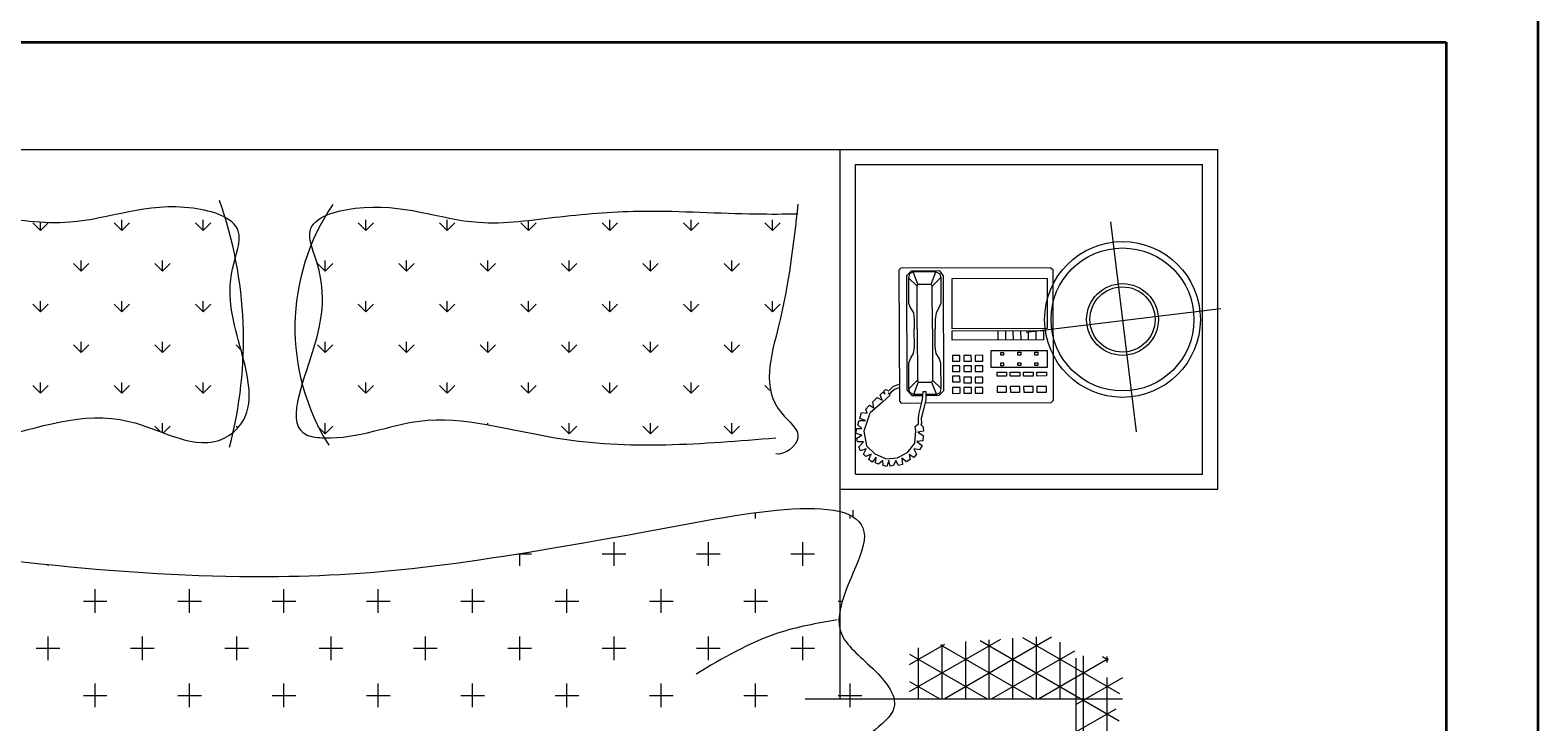
# Model space of a CAD drawing. Units: inches. Extents: x 3731 to 4318, y 1310 to 2388.
# Tile 55 of 57: x 4157 to 4239, y 2296 to 2334. Entities that reach past the tile are written whole.
import ezdxf

# ---------------------------------------------------------------- set-up
doc = ezdxf.new("R2010")
doc.units = ezdxf.units.IN
for name, color, linetype, lineweight in [('A-ANNO-DIMS', 2, 'Continuous', 18), ('A-FURN', 8, 'Continuous', 13), ('A-WALL', 7, 'Continuous', 35)]:
    doc.layers.add(name, color=color, linetype=linetype, lineweight=lineweight)
doc.styles.get("Standard").update_dxf_attribs({"font": 'arial.ttf'})
doc.dimstyles.get("Standard").update_dxf_attribs({"dimtxt": 0.18, "dimasz": 0.18, "dimexe": 0.18, "dimexo": 0.0625, "dimgap": 0.09, "dimtad": 0, "dimtih": 1, "dimtoh": 1, "dimdec": 4, "dimzin": 0, "dimdsep": 46, "dimtxsty": 'Standard', "dimcen": 0.09, "dimadec": 0, "dimazin": 0, "dimtfac": 1, "dimtdec": 4, "dimtofl": 0, "dimtmove": 0, "dimatfit": 3, "dimfxl": 1, "dimtolj": 1, "dimtzin": 0, "dimarcsym": 0})

# ---------------------------------------------------------------- blocks, each defined once
blk = doc.blocks.new('A$C200C7901')
for p, q in [((0.5, 2.3334), (2, 2.3334)), ((2, 2.3334), (2.5, 2.3334)), ((2, 1.6055), (2, 2.3334)), ((2.5, 1.8834), (2.5, 2.3334)), ((0.9943, 2.1721), (0.9842, 2.1822)), ((0.9943, 2.1721), (0.9842, 2.1822)), ((1.3176, 2.1721), (1.3075, 2.1822)), ((1.3176, 2.1721), (1.3075, 2.1822)), ((0.9943, 2.0643), (0.9842, 2.0744)), ((0.9943, 2.0643), (0.9842, 2.0744)), ((1.206, 2.0681), (1.1997, 2.0744)), ((1.206, 2.0681), (1.1997, 2.0744)), ((1.2019, 1.9645), (1.1997, 1.9666)), ((1.2019, 1.9645), (1.1997, 1.9666)), ((2, 1.8834), (2.5, 1.8834)), ((2.0129, 1.8445), (2.0129, 1.849)), ((2.0129, 1.8445), (2.0129, 1.849)), ((2.0171, 1.8467), (2.0171, 1.8556)), ((2.0171, 1.8467), (2.0171, 1.8556)), ((1.1379, 1.7195), (1.1379, 1.7508)), ((1.1222, 1.7352), (1.1535, 1.7352)), ((1.9972, 1.7352), (2.0027, 1.7352)), ((1.9972, 1.7352), (2.0027, 1.7352)), ((2, 1.6963), (2, 1.7248)), ((2, 1.6963), (2, 1.7248)), ((2.3121, 1.6596), (2.3121, 0.0201)), ((1.0129, 1.5945), (1.0129, 1.6258)), ((1.0129, 1.5945), (1.0129, 1.6258)), ((1.9533, 1.6055), (2.3741, 1.6055)), ((1.9533, 1.6055), (2.3741, 1.6055))]:
    blk.add_line(p, q)
at = {"linetype": 'ByBlock'}
for p, q in [((2.02, 2.3134), (2.48, 2.3134)), ((2.02, 1.9034), (2.02, 2.3134)), ((2.48, 1.9034), (2.48, 2.3134)), ((1.0482, 2.2259), (1.0482, 2.2402)), ((1.0482, 2.2259), (1.0482, 2.2402)), ((1.1559, 2.2259), (1.1559, 2.2402)), ((1.1559, 2.2259), (1.1559, 2.2402)), ((1.3714, 2.2259), (1.3714, 2.2402)), ((1.3714, 2.2259), (1.3714, 2.2402)), ((1.4792, 2.2259), (1.4792, 2.2402)), ((1.4792, 2.2259), (1.4792, 2.2402)), ((1.587, 2.2259), (1.587, 2.2393)), ((1.587, 2.2259), (1.587, 2.2393)), ((1.6947, 2.2259), (1.6947, 2.2402)), ((1.6947, 2.2259), (1.6947, 2.2402)), ((1.8025, 2.2259), (1.8025, 2.2402)), ((1.8025, 2.2259), (1.8025, 2.2402)), ((1.9103, 2.2259), (1.9103, 2.2402)), ((1.9103, 2.2259), (1.9103, 2.2402)), ((2.3581, 2.2373), (2.3919, 1.9595)), ((0.9404, 2.2259), (0.9303, 2.236)), ((0.9404, 2.2259), (0.9303, 2.236)), ((0.9404, 2.2259), (0.9404, 2.2369)), ((0.9404, 2.2259), (0.9404, 2.2369)), ((0.9404, 2.2259), (0.9505, 2.236)), ((0.9404, 2.2259), (0.9505, 2.236)), ((1.0482, 2.2259), (1.0381, 2.236)), ((1.0482, 2.2259), (1.0381, 2.236)), ((1.0482, 2.2259), (1.0583, 2.236)), ((1.0482, 2.2259), (1.0583, 2.236)), ((1.1559, 2.2259), (1.1458, 2.236)), ((1.1559, 2.2259), (1.1458, 2.236)), ((1.1559, 2.2259), (1.166, 2.236)), ((1.1559, 2.2259), (1.166, 2.236)), ((1.3714, 2.2259), (1.3613, 2.236)), ((1.3714, 2.2259), (1.3613, 2.236)), ((1.3714, 2.2259), (1.3815, 2.236)), ((1.3714, 2.2259), (1.3815, 2.236)), ((1.4792, 2.2259), (1.4691, 2.236)), ((1.4792, 2.2259), (1.4691, 2.236)), ((1.4792, 2.2259), (1.4893, 2.236)), ((1.4792, 2.2259), (1.4893, 2.236)), ((1.587, 2.2259), (1.5769, 2.236)), ((1.587, 2.2259), (1.5769, 2.236)), ((1.587, 2.2259), (1.5971, 2.236)), ((1.587, 2.2259), (1.5971, 2.236)), ((1.6947, 2.2259), (1.6846, 2.236)), ((1.6947, 2.2259), (1.6846, 2.236)), ((1.6947, 2.2259), (1.7048, 2.236)), ((1.6947, 2.2259), (1.7048, 2.236)), ((1.8025, 2.2259), (1.7924, 2.236)), ((1.8025, 2.2259), (1.7924, 2.236)), ((1.8025, 2.2259), (1.8126, 2.236)), ((1.8025, 2.2259), (1.8126, 2.236)), ((1.9103, 2.2259), (1.9002, 2.236)), ((1.9103, 2.2259), (1.9002, 2.236)), ((1.9103, 2.2259), (1.9204, 2.236)), ((1.9103, 2.2259), (1.9204, 2.236)), ((0.9943, 2.172), (0.9943, 2.1863)), ((0.9943, 2.172), (0.9943, 2.1863)), ((0.9943, 2.1721), (1.0044, 2.1822)), ((0.9943, 2.1721), (1.0044, 2.1822)), ((1.102, 2.1721), (1.0919, 2.1822)), ((1.102, 2.1721), (1.0919, 2.1822)), ((1.102, 2.172), (1.102, 2.1863)), ((1.102, 2.172), (1.102, 2.1863)), ((1.102, 2.1721), (1.1121, 2.1822)), ((1.102, 2.1721), (1.1121, 2.1822)), ((1.3176, 2.172), (1.3176, 2.1863)), ((1.3176, 2.172), (1.3176, 2.1863)), ((1.3176, 2.1721), (1.3277, 2.1822)), ((1.3176, 2.1721), (1.3277, 2.1822)), ((1.4253, 2.1721), (1.4152, 2.1822)), ((1.4253, 2.1721), (1.4152, 2.1822)), ((1.4253, 2.172), (1.4253, 2.1863)), ((1.4253, 2.172), (1.4253, 2.1863)), ((1.4253, 2.1721), (1.4354, 2.1822)), ((1.4253, 2.1721), (1.4354, 2.1822)), ((1.5331, 2.1721), (1.523, 2.1822)), ((1.5331, 2.1721), (1.523, 2.1822)), ((1.5331, 2.172), (1.5331, 2.1863)), ((1.5331, 2.172), (1.5331, 2.1863)), ((1.5331, 2.1721), (1.5432, 2.1822)), ((1.5331, 2.1721), (1.5432, 2.1822)), ((1.6409, 2.1721), (1.6308, 2.1822)), ((1.6409, 2.1721), (1.6308, 2.1822)), ((1.6408, 2.172), (1.6408, 2.1863)), ((1.6408, 2.172), (1.6408, 2.1863)), ((1.6409, 2.1721), (1.651, 2.1822)), ((1.6409, 2.1721), (1.651, 2.1822)), ((1.7486, 2.1721), (1.7385, 2.1822)), ((1.7486, 2.1721), (1.7385, 2.1822)), ((1.7486, 2.172), (1.7486, 2.1863)), ((1.7486, 2.172), (1.7486, 2.1863)), ((1.7486, 2.1721), (1.7587, 2.1822)), ((1.7486, 2.1721), (1.7587, 2.1822)), ((1.8564, 2.1721), (1.8463, 2.1822)), ((1.8564, 2.1721), (1.8463, 2.1822)), ((1.8564, 2.172), (1.8564, 2.1863)), ((1.8564, 2.172), (1.8564, 2.1863)), ((1.8564, 2.1721), (1.8665, 2.1822)), ((1.8564, 2.1721), (1.8665, 2.1822)), ((2.0802, 2.176), (2.0777, 2.1734)), ((2.0777, 2.1734), (2.0783, 1.9999)), ((2.2789, 2.1766), (2.0802, 2.176)), ((2.0941, 2.1722), (2.0878, 2.1659)), ((2.0878, 2.1659), (2.0883, 2.015)), ((2.0915, 2.1685), (2.0903, 2.1634)), ((2.0903, 2.1634), (2.1017, 2.1521)), ((2.0903, 2.1634), (2.0904, 2.1295)), ((2.0966, 2.171), (2.0915, 2.1685)), ((2.1318, 2.1724), (2.0941, 2.1722)), ((2.1267, 2.1711), (2.0966, 2.171)), ((2.1029, 2.1547), (2.0966, 2.171)), ((2.1205, 2.1547), (2.1267, 2.1711)), ((2.1331, 2.1636), (2.1218, 2.1522)), ((2.1267, 2.1711), (2.1318, 2.1686)), ((2.1368, 2.1661), (2.1318, 2.1724)), ((2.1318, 2.1686), (2.1331, 2.1636)), ((2.1331, 2.1636), (2.1332, 2.1296)), ((2.1373, 2.014), (2.1368, 2.1661)), ((2.1481, 2.1624), (2.2739, 2.1628)), ((2.1484, 2.0957), (2.1481, 2.1624)), ((2.2739, 2.1628), (2.2741, 2.0961)), ((2.2789, 2.1766), (2.2814, 2.1741)), ((2.2814, 2.1741), (2.282, 2.0006)), ((2.1017, 2.1521), (2.1029, 2.1547)), ((2.1019, 2.0956), (2.1017, 2.1521)), ((2.1029, 2.1547), (2.1205, 2.1547)), ((2.1218, 2.1522), (2.1205, 2.1547)), ((2.122, 2.0956), (2.1218, 2.1522)), ((0.9404, 2.1182), (0.9303, 2.1283)), ((0.9404, 2.1182), (0.9303, 2.1283)), ((0.9404, 2.1182), (0.9404, 2.1325)), ((0.9404, 2.1182), (0.9404, 2.1325)), ((0.9404, 2.1182), (0.9505, 2.1283)), ((0.9404, 2.1182), (0.9505, 2.1283)), ((1.0482, 2.1182), (1.0381, 2.1283)), ((1.0482, 2.1182), (1.0381, 2.1283)), ((1.0482, 2.1182), (1.0482, 2.1325)), ((1.0482, 2.1182), (1.0482, 2.1325)), ((1.0482, 2.1182), (1.0583, 2.1283)), ((1.0482, 2.1182), (1.0583, 2.1283)), ((1.1559, 2.1182), (1.1458, 2.1283)), ((1.1559, 2.1182), (1.1458, 2.1283)), ((1.1559, 2.1182), (1.1559, 2.1325)), ((1.1559, 2.1182), (1.1559, 2.1325)), ((1.1559, 2.1182), (1.166, 2.1283)), ((1.1559, 2.1182), (1.166, 2.1283)), ((1.3714, 2.1182), (1.3613, 2.1283)), ((1.3714, 2.1182), (1.3613, 2.1283)), ((1.3714, 2.1182), (1.3714, 2.1325)), ((1.3714, 2.1182), (1.3714, 2.1325)), ((1.3714, 2.1182), (1.3815, 2.1283)), ((1.3714, 2.1182), (1.3815, 2.1283)), ((1.4792, 2.1182), (1.4691, 2.1283)), ((1.4792, 2.1182), (1.4691, 2.1283)), ((1.4792, 2.1182), (1.4792, 2.1325)), ((1.4792, 2.1182), (1.4792, 2.1325)), ((1.4792, 2.1182), (1.4893, 2.1283)), ((1.4792, 2.1182), (1.4893, 2.1283)), ((1.587, 2.1182), (1.5769, 2.1283)), ((1.587, 2.1182), (1.5769, 2.1283)), ((1.587, 2.1182), (1.587, 2.1325)), ((1.587, 2.1182), (1.587, 2.1325)), ((1.587, 2.1182), (1.5971, 2.1283)), ((1.587, 2.1182), (1.5971, 2.1283)), ((1.6947, 2.1182), (1.6846, 2.1283)), ((1.6947, 2.1182), (1.6846, 2.1283)), ((1.6947, 2.1182), (1.6947, 2.1325)), ((1.6947, 2.1182), (1.6947, 2.1325)), ((1.6947, 2.1182), (1.7048, 2.1283)), ((1.6947, 2.1182), (1.7048, 2.1283)), ((1.8025, 2.1182), (1.7924, 2.1283)), ((1.8025, 2.1182), (1.7924, 2.1283)), ((1.8025, 2.1182), (1.8025, 2.1325)), ((1.8025, 2.1182), (1.8025, 2.1325)), ((1.8025, 2.1182), (1.8126, 2.1283)), ((1.8025, 2.1182), (1.8126, 2.1283)), ((1.9103, 2.1182), (1.9002, 2.1283)), ((1.9103, 2.1182), (1.9002, 2.1283)), ((1.9103, 2.1182), (1.9103, 2.1325)), ((1.9103, 2.1182), (1.9103, 2.1325)), ((1.9103, 2.1182), (1.9204, 2.1283)), ((1.9103, 2.1182), (1.9204, 2.1283)), ((2.0904, 2.1295), (2.093, 2.1232)), ((2.093, 2.1232), (2.0968, 2.1169)), ((2.1307, 2.1233), (2.1269, 2.117)), ((2.1332, 2.1296), (2.1307, 2.1233)), ((2.2464, 2.0911), (2.5044, 2.1228)), ((2.0968, 2.1169), (2.098, 2.1081)), ((2.098, 2.1081), (2.0981, 2.0956)), ((2.1269, 2.117), (2.1257, 2.1082)), ((2.1257, 2.1082), (2.1257, 2.0956)), ((0.9943, 2.0643), (0.9943, 2.0786)), ((0.9943, 2.0643), (0.9943, 2.0786)), ((1.102, 2.0643), (1.102, 2.0786)), ((1.102, 2.0643), (1.102, 2.0786)), ((1.3176, 2.0643), (1.3176, 2.0786)), ((1.3176, 2.0643), (1.3176, 2.0786)), ((1.4253, 2.0643), (1.4253, 2.0786)), ((1.4253, 2.0643), (1.4253, 2.0786)), ((1.5331, 2.0643), (1.5331, 2.0786)), ((1.5331, 2.0643), (1.5331, 2.0786)), ((1.6408, 2.0643), (1.6408, 2.0786)), ((1.6408, 2.0643), (1.6408, 2.0786)), ((1.7486, 2.0643), (1.7486, 2.0786)), ((1.7486, 2.0643), (1.7486, 2.0786)), ((1.8564, 2.0643), (1.8564, 2.0786)), ((1.8564, 2.0643), (1.8564, 2.0786)), ((2.0982, 2.0717), (2.0981, 2.0956)), ((2.1019, 2.0956), (2.1021, 2.0277)), ((2.122, 2.0956), (2.1222, 2.0277)), ((2.1258, 2.0718), (2.1257, 2.0956)), ((2.2741, 2.0961), (2.1484, 2.0957)), ((2.1484, 2.0932), (2.2691, 2.0936)), ((2.1484, 2.0806), (2.1484, 2.0932)), ((2.2691, 2.081), (2.1484, 2.0806)), ((2.2087, 2.0934), (2.2088, 2.0808)), ((2.2188, 2.0934), (2.2188, 2.0809)), ((2.2288, 2.0935), (2.2289, 2.0809)), ((2.2389, 2.0935), (2.239, 2.0809)), ((2.249, 2.0935), (2.249, 2.081)), ((2.259, 2.0936), (2.2591, 2.081)), ((2.2691, 2.0936), (2.2691, 2.081)), ((0.9943, 2.0643), (1.0044, 2.0744)), ((0.9943, 2.0643), (1.0044, 2.0744)), ((1.102, 2.0643), (1.0919, 2.0744)), ((1.102, 2.0643), (1.0919, 2.0744)), ((1.102, 2.0643), (1.1121, 2.0744)), ((1.102, 2.0643), (1.1121, 2.0744)), ((1.3176, 2.0643), (1.3075, 2.0744)), ((1.3176, 2.0643), (1.3075, 2.0744)), ((1.3176, 2.0643), (1.3277, 2.0744)), ((1.3176, 2.0643), (1.3277, 2.0744)), ((1.4253, 2.0643), (1.4152, 2.0744)), ((1.4253, 2.0643), (1.4152, 2.0744)), ((1.4253, 2.0643), (1.4354, 2.0744)), ((1.4253, 2.0643), (1.4354, 2.0744)), ((1.5331, 2.0643), (1.523, 2.0744)), ((1.5331, 2.0643), (1.523, 2.0744)), ((1.5331, 2.0643), (1.5432, 2.0744)), ((1.5331, 2.0643), (1.5432, 2.0744)), ((1.6409, 2.0643), (1.6308, 2.0744)), ((1.6409, 2.0643), (1.6308, 2.0744)), ((1.6409, 2.0643), (1.651, 2.0744)), ((1.6409, 2.0643), (1.651, 2.0744)), ((1.7486, 2.0643), (1.7385, 2.0744)), ((1.7486, 2.0643), (1.7385, 2.0744)), ((1.7486, 2.0643), (1.7587, 2.0744)), ((1.7486, 2.0643), (1.7587, 2.0744)), ((1.8564, 2.0643), (1.8463, 2.0744)), ((1.8564, 2.0643), (1.8463, 2.0744)), ((1.8564, 2.0643), (1.8665, 2.0744)), ((1.8564, 2.0643), (1.8665, 2.0744)), ((2.0932, 2.0566), (2.0969, 2.0629)), ((2.0969, 2.0629), (2.0982, 2.0717)), ((2.1271, 2.063), (2.1258, 2.0718)), ((2.1309, 2.0567), (2.1271, 2.063)), ((2.1586, 2.0606), (2.1485, 2.0605)), ((2.1485, 2.0605), (2.1485, 2.053)), ((2.1586, 2.053), (2.1586, 2.0606)), ((2.1636, 2.0606), (2.1636, 2.053)), ((2.1736, 2.0606), (2.1636, 2.0606)), ((2.1737, 2.0531), (2.1736, 2.0606)), ((2.1887, 2.0607), (2.1787, 2.0606)), ((2.1787, 2.0606), (2.1787, 2.0531)), ((2.1888, 2.0531), (2.1887, 2.0607)), ((2.2, 2.067), (2.2742, 2.0672)), ((2.2001, 2.0443), (2.2, 2.067)), ((2.2126, 2.0645), (2.2164, 2.0645)), ((2.2126, 2.0607), (2.2126, 2.0645)), ((2.2164, 2.0607), (2.2126, 2.0607)), ((2.2164, 2.0645), (2.2164, 2.0607)), ((2.2352, 2.0646), (2.239, 2.0646)), ((2.2352, 2.0608), (2.2352, 2.0646)), ((2.239, 2.0608), (2.2352, 2.0608)), ((2.239, 2.0646), (2.239, 2.0608)), ((2.2579, 2.0609), (2.2579, 2.0647)), ((2.2579, 2.0647), (2.2616, 2.0647)), ((2.2616, 2.0609), (2.2579, 2.0609)), ((2.2616, 2.0647), (2.2616, 2.0609)), ((2.2742, 2.0672), (2.2743, 2.0446)), ((2.0907, 2.0503), (2.0932, 2.0566)), ((2.0908, 2.0163), (2.0907, 2.0503)), ((2.1334, 2.0504), (2.1309, 2.0567)), ((2.1336, 2.0165), (2.1334, 2.0504)), ((2.1485, 2.053), (2.1586, 2.053)), ((2.1485, 2.0467), (2.1486, 2.0391)), ((2.1586, 2.0467), (2.1485, 2.0467)), ((2.1486, 2.0391), (2.1586, 2.0392)), ((2.1586, 2.0392), (2.1586, 2.0467)), ((2.1636, 2.053), (2.1737, 2.0531)), ((2.1737, 2.0468), (2.1636, 2.0467)), ((2.1636, 2.0467), (2.1637, 2.0392)), ((2.1637, 2.0392), (2.1737, 2.0392)), ((2.1737, 2.0392), (2.1737, 2.0468)), ((2.1787, 2.0531), (2.1888, 2.0531)), ((2.1787, 2.0468), (2.1787, 2.0392)), ((2.1888, 2.0468), (2.1787, 2.0468)), ((2.1787, 2.0392), (2.1888, 2.0393)), ((2.1888, 2.0393), (2.1888, 2.0468)), ((2.2743, 2.0446), (2.2001, 2.0443)), ((2.2077, 2.0331), (2.2077, 2.0381)), ((2.2077, 2.0381), (2.2202, 2.0381)), ((2.2126, 2.0507), (2.2164, 2.0507)), ((2.2127, 2.0469), (2.2126, 2.0507)), ((2.2164, 2.0469), (2.2127, 2.0469)), ((2.2164, 2.0507), (2.2164, 2.0469)), ((2.2202, 2.0381), (2.2203, 2.0331)), ((2.2253, 2.0381), (2.2378, 2.0382)), ((2.2253, 2.0331), (2.2253, 2.0381)), ((2.2353, 2.0508), (2.2391, 2.0508)), ((2.2353, 2.047), (2.2353, 2.0508)), ((2.2391, 2.047), (2.2353, 2.047)), ((2.2378, 2.0382), (2.2379, 2.0332)), ((2.2391, 2.0508), (2.2391, 2.047)), ((2.2429, 2.0332), (2.2429, 2.0382)), ((2.2429, 2.0382), (2.2554, 2.0382)), ((2.2554, 2.0382), (2.2555, 2.0332)), ((2.2579, 2.0508), (2.2617, 2.0508)), ((2.2579, 2.0471), (2.2579, 2.0508)), ((2.2617, 2.0471), (2.2579, 2.0471)), ((2.2605, 2.0332), (2.2605, 2.0383)), ((2.2605, 2.0383), (2.273, 2.0383)), ((2.2617, 2.0508), (2.2617, 2.0471)), ((2.273, 2.0383), (2.2731, 2.0333)), ((0.9404, 2.0104), (0.9303, 2.0205)), ((0.9404, 2.0104), (0.9303, 2.0205)), ((0.9404, 2.0104), (0.9404, 2.0247)), ((0.9404, 2.0104), (0.9404, 2.0247)), ((0.9404, 2.0104), (0.9505, 2.0205)), ((0.9404, 2.0104), (0.9505, 2.0205)), ((1.0482, 2.0104), (1.0381, 2.0205)), ((1.0482, 2.0104), (1.0381, 2.0205)), ((1.0482, 2.0104), (1.0482, 2.0247)), ((1.0482, 2.0104), (1.0482, 2.0247)), ((1.0482, 2.0104), (1.0583, 2.0205)), ((1.0482, 2.0104), (1.0583, 2.0205)), ((1.1559, 2.0104), (1.1458, 2.0205)), ((1.1559, 2.0104), (1.1458, 2.0205)), ((1.1559, 2.0104), (1.1559, 2.0247)), ((1.1559, 2.0104), (1.1559, 2.0247)), ((1.1559, 2.0104), (1.166, 2.0205)), ((1.1559, 2.0104), (1.166, 2.0205)), ((1.3714, 2.0104), (1.3613, 2.0205)), ((1.3714, 2.0104), (1.3613, 2.0205)), ((1.3714, 2.0104), (1.3714, 2.0247)), ((1.3714, 2.0104), (1.3714, 2.0247)), ((1.3714, 2.0104), (1.3815, 2.0205)), ((1.3714, 2.0104), (1.3815, 2.0205)), ((1.4792, 2.0104), (1.4691, 2.0205)), ((1.4792, 2.0104), (1.4691, 2.0205)), ((1.4792, 2.0104), (1.4792, 2.0247)), ((1.4792, 2.0104), (1.4792, 2.0247)), ((1.4792, 2.0104), (1.4893, 2.0205)), ((1.4792, 2.0104), (1.4893, 2.0205)), ((1.587, 2.0104), (1.5769, 2.0205)), ((1.587, 2.0104), (1.5769, 2.0205)), ((1.587, 2.0104), (1.587, 2.0247)), ((1.587, 2.0104), (1.587, 2.0247)), ((1.587, 2.0104), (1.5971, 2.0205)), ((1.587, 2.0104), (1.5971, 2.0205)), ((1.6947, 2.0104), (1.6846, 2.0205)), ((1.6947, 2.0104), (1.6846, 2.0205)), ((1.6947, 2.0104), (1.6947, 2.0247)), ((1.6947, 2.0104), (1.6947, 2.0247)), ((1.6947, 2.0104), (1.7048, 2.0205)), ((1.6947, 2.0104), (1.7048, 2.0205)), ((1.8025, 2.0104), (1.7924, 2.0205)), ((1.8025, 2.0104), (1.7924, 2.0205)), ((1.8025, 2.0104), (1.8025, 2.0247)), ((1.8025, 2.0104), (1.8025, 2.0247)), ((1.8025, 2.0104), (1.8126, 2.0205)), ((1.8025, 2.0104), (1.8126, 2.0205)), ((1.9068, 2.0139), (1.9002, 2.0205)), ((1.9068, 2.0139), (1.9002, 2.0205)), ((2.0671, 2.0162), (2.0707, 2.0197)), ((2.0707, 2.0197), (2.0782, 2.0226)), ((2.0782, 2.0175), (2.0727, 2.016)), ((2.0908, 2.0163), (2.1021, 2.0277)), ((2.1034, 2.0252), (2.0971, 2.0088)), ((2.1021, 2.0277), (2.1034, 2.0252)), ((2.1034, 2.0252), (2.121, 2.0252)), ((2.1222, 2.0277), (2.121, 2.0252)), ((2.121, 2.0252), (2.1273, 2.0089)), ((2.1336, 2.0165), (2.1222, 2.0277)), ((2.1586, 2.0329), (2.1486, 2.0329)), ((2.1486, 2.0329), (2.1486, 2.0253)), ((2.1486, 2.0253), (2.1587, 2.0253)), ((2.1587, 2.0178), (2.1486, 2.0178)), ((2.1486, 2.0178), (2.1487, 2.0102)), ((2.1587, 2.0253), (2.1586, 2.0329)), ((2.1587, 2.0103), (2.1587, 2.0178)), ((2.1637, 2.0317), (2.1637, 2.0241)), ((2.1737, 2.0317), (2.1637, 2.0317)), ((2.1637, 2.0241), (2.1738, 2.0241)), ((2.1738, 2.0179), (2.1637, 2.0178)), ((2.1637, 2.0178), (2.1638, 2.0103)), ((2.1738, 2.0241), (2.1737, 2.0317)), ((2.1738, 2.0103), (2.1738, 2.0179)), ((2.1788, 2.0317), (2.1788, 2.0242)), ((2.1888, 2.0317), (2.1788, 2.0317)), ((2.1788, 2.0242), (2.1889, 2.0242)), ((2.1788, 2.0179), (2.1788, 2.0103)), ((2.1889, 2.0179), (2.1788, 2.0179)), ((2.1889, 2.0242), (2.1888, 2.0317)), ((2.1889, 2.0104), (2.1889, 2.0179)), ((2.2203, 2.0331), (2.2077, 2.0331)), ((2.2203, 2.0193), (2.2077, 2.0192)), ((2.2077, 2.0192), (2.2078, 2.0117)), ((2.2203, 2.0117), (2.2203, 2.0193)), ((2.2379, 2.0332), (2.2253, 2.0331)), ((2.2379, 2.0193), (2.2253, 2.0193)), ((2.2253, 2.0193), (2.2254, 2.0117)), ((2.2379, 2.0118), (2.2379, 2.0193)), ((2.2555, 2.0332), (2.2429, 2.0332)), ((2.2555, 2.0194), (2.2429, 2.0193)), ((2.2429, 2.0193), (2.243, 2.0118)), ((2.2555, 2.0118), (2.2555, 2.0194)), ((2.2731, 2.0333), (2.2605, 2.0332)), ((2.2605, 2.0194), (2.2606, 2.0119)), ((2.2731, 2.0194), (2.2605, 2.0194)), ((2.2731, 2.0119), (2.2731, 2.0194)), ((2.0561, 1.9986), (2.0396, 1.9844)), ((2.0431, 1.999), (2.0488, 2.0046)), ((2.0444, 1.9911), (2.0431, 1.999)), ((2.0488, 2.0046), (2.0557, 2.0011)), ((2.053, 2.0084), (2.0563, 2.0119)), ((2.0557, 2.0011), (2.053, 2.0084)), ((2.0663, 2.0077), (2.0561, 1.9986)), ((2.0563, 2.0119), (2.0594, 2.0095)), ((2.0576, 2.0133), (2.0598, 2.0155)), ((2.0594, 2.0095), (2.0576, 2.0133)), ((2.0598, 2.0155), (2.0645, 2.0137)), ((2.0663, 2.0102), (2.0636, 2.0104)), ((2.0636, 2.0104), (2.0663, 2.0077)), ((2.0645, 2.0137), (2.0671, 2.0162)), ((2.0676, 2.012), (2.0663, 2.0102)), ((2.0727, 2.016), (2.0676, 2.012)), ((2.0783, 1.9999), (2.0808, 1.9974)), ((2.0808, 1.9974), (2.1079, 1.9975)), ((2.0883, 2.015), (2.0946, 2.0075)), ((2.0921, 2.0113), (2.0908, 2.0163)), ((2.0971, 2.0088), (2.0921, 2.0113)), ((2.0946, 2.0075), (2.1093, 2.0076)), ((2.1094, 2.0088), (2.0971, 2.0088)), ((2.1072, 1.9944), (2.109, 2.0025)), ((2.109, 2.0025), (2.1097, 2.0126)), ((2.1097, 2.0126), (2.1135, 2.0126)), ((2.1133, 2.0018), (2.1103, 1.989)), ((2.1123, 1.9975), (2.2795, 1.9981)), ((2.1135, 2.0126), (2.1133, 2.0018)), ((2.1273, 2.0089), (2.1134, 2.0088)), ((2.1134, 2.0076), (2.1311, 2.0077)), ((2.1273, 2.0089), (2.1323, 2.0114)), ((2.1311, 2.0077), (2.1373, 2.014)), ((2.1323, 2.0114), (2.1336, 2.0165)), ((2.1487, 2.0102), (2.1587, 2.0103)), ((2.1638, 2.0103), (2.1738, 2.0103)), ((2.1788, 2.0103), (2.1889, 2.0104)), ((2.2078, 2.0117), (2.2203, 2.0117)), ((2.2254, 2.0117), (2.2379, 2.0118)), ((2.243, 2.0118), (2.2555, 2.0118)), ((2.2606, 2.0119), (2.2731, 2.0119)), ((2.282, 2.0006), (2.2795, 1.9981)), ((2.0259, 1.977), (2.0281, 1.9847)), ((2.0281, 1.9847), (2.0358, 1.9839)), ((2.0393, 1.984), (2.031, 1.96)), ((2.0338, 1.9895), (2.0386, 1.9946)), ((2.0358, 1.9839), (2.0338, 1.9895)), ((2.0386, 1.9946), (2.0444, 1.9911)), ((2.1035, 1.9763), (2.1042, 1.9824)), ((2.1042, 1.9824), (2.1072, 1.9944)), ((2.1103, 1.989), (2.1073, 1.9771)), ((1.0993, 1.9593), (1.0919, 1.9666)), ((1.0993, 1.9593), (1.0919, 1.9666)), ((1.102, 1.9583), (1.102, 1.9708)), ((1.102, 1.9583), (1.102, 1.9708)), ((1.1033, 1.9578), (1.1121, 1.9666)), ((1.1033, 1.9578), (1.1121, 1.9666)), ((1.3176, 1.9565), (1.3075, 1.9666)), ((1.3176, 1.9565), (1.3075, 1.9666)), ((1.3176, 1.9565), (1.3176, 1.9708)), ((1.3176, 1.9565), (1.3176, 1.9708)), ((1.3176, 1.9565), (1.3277, 1.9666)), ((1.3176, 1.9565), (1.3277, 1.9666)), ((1.4253, 1.9703), (1.4253, 1.9708)), ((1.4253, 1.9703), (1.4253, 1.9708)), ((1.5331, 1.9683), (1.5331, 1.9708)), ((1.5331, 1.9683), (1.5331, 1.9708)), ((1.543, 1.9665), (1.5432, 1.9666)), ((1.543, 1.9665), (1.5432, 1.9666)), ((1.6409, 1.9565), (1.6308, 1.9666)), ((1.6409, 1.9565), (1.6308, 1.9666)), ((1.6408, 1.9565), (1.6408, 1.9708)), ((1.6408, 1.9565), (1.6408, 1.9708)), ((1.6409, 1.9565), (1.651, 1.9666)), ((1.6409, 1.9565), (1.651, 1.9666)), ((1.7486, 1.9565), (1.7385, 1.9666)), ((1.7486, 1.9565), (1.7385, 1.9666)), ((1.7486, 1.9565), (1.7486, 1.9708)), ((1.7486, 1.9565), (1.7486, 1.9708)), ((1.7486, 1.9565), (1.7587, 1.9666)), ((1.7486, 1.9565), (1.7587, 1.9666)), ((1.8564, 1.9565), (1.8463, 1.9666)), ((1.8564, 1.9565), (1.8463, 1.9666)), ((1.8564, 1.9565), (1.8564, 1.9708)), ((1.8564, 1.9565), (1.8564, 1.9708)), ((1.8564, 1.9565), (1.8665, 1.9666)), ((1.8564, 1.9565), (1.8665, 1.9666)), ((2.0206, 1.9572), (2.0218, 1.9635)), ((2.0218, 1.9635), (2.0287, 1.9636)), ((2.0234, 1.9686), (2.0251, 1.9745)), ((2.0287, 1.9636), (2.0234, 1.9686)), ((2.0251, 1.9745), (2.0333, 1.9743)), ((2.0333, 1.9743), (2.0259, 1.977)), ((2.031, 1.96), (2.0346, 1.9409)), ((2.099, 1.9444), (2.1002, 1.9605)), ((2.0992, 1.9663), (2.1038, 1.9697)), ((2.1002, 1.9605), (2.0992, 1.9663)), ((2.1101, 1.96), (2.1028, 1.9587)), ((2.1028, 1.9587), (2.1099, 1.9544)), ((2.1038, 1.9697), (2.1035, 1.9763)), ((2.1076, 1.9704), (2.1068, 1.9689)), ((2.1068, 1.9689), (2.1096, 1.9661)), ((2.1073, 1.9771), (2.1076, 1.9704)), ((2.1096, 1.9661), (2.1101, 1.96)), ((2.0285, 1.9549), (2.0206, 1.9572)), ((2.0219, 1.9511), (2.0285, 1.9549)), ((2.0229, 1.946), (2.0219, 1.9511)), ((2.0308, 1.9462), (2.0229, 1.946)), ((2.0247, 1.9394), (2.0308, 1.9462)), ((2.0268, 1.9343), (2.0247, 1.9394)), ((2.0346, 1.9409), (2.0459, 1.93)), ((2.0894, 1.9322), (2.099, 1.9444)), ((2.1094, 1.9475), (2.1013, 1.9467)), ((2.1013, 1.9467), (2.1084, 1.9412)), ((2.1084, 1.9412), (2.1051, 1.9353)), ((2.1099, 1.9544), (2.1094, 1.9475)), ((2.0341, 1.9366), (2.0268, 1.9343)), ((2.0306, 1.9297), (2.0341, 1.9366)), ((2.0339, 1.9267), (2.0306, 1.9297)), ((2.041, 1.9297), (2.0339, 1.9267)), ((2.038, 1.9228), (2.041, 1.9297)), ((2.0421, 1.9193), (2.038, 1.9228)), ((2.0474, 1.9259), (2.0421, 1.9193)), ((2.0459, 1.93), (2.0607, 1.9237)), ((2.0467, 1.9183), (2.0474, 1.9259)), ((2.0508, 1.9163), (2.0467, 1.9183)), ((2.0566, 1.9214), (2.0508, 1.9163)), ((2.0569, 1.9145), (2.0566, 1.9214)), ((2.0607, 1.9237), (2.0759, 1.925)), ((2.0645, 1.9214), (2.0617, 1.9133)), ((2.0663, 1.914), (2.0645, 1.9214)), ((2.0736, 1.9214), (2.0706, 1.9146)), ((2.077, 1.9146), (2.0736, 1.9214)), ((2.0759, 1.925), (2.0894, 1.9322)), ((2.0876, 1.9195), (2.0815, 1.9245)), ((2.0815, 1.9245), (2.0823, 1.9161)), ((2.0925, 1.9225), (2.0876, 1.9195)), ((2.0973, 1.9251), (2.0914, 1.9294)), ((2.0914, 1.9294), (2.0925, 1.9225)), ((2.1011, 1.9297), (2.0973, 1.9251)), ((2.1051, 1.9353), (2.0975, 1.9368)), ((2.0975, 1.9368), (2.1011, 1.9297)), ((2.02, 1.9034), (2.48, 1.9034)), ((2.0617, 1.9133), (2.0569, 1.9145)), ((2.0706, 1.9146), (2.0663, 1.914)), ((2.0823, 1.9161), (2.077, 1.9146)), ((1.8879, 1.8445), (1.8879, 1.8523)), ((1.8879, 1.8445), (1.8879, 1.8523)), ((1.5754, 1.782), (1.5754, 1.7981)), ((1.5754, 1.782), (1.5754, 1.7981)), ((1.7004, 1.782), (1.7004, 1.8133)), ((1.7004, 1.782), (1.7004, 1.8133)), ((1.8254, 1.782), (1.8254, 1.8133)), ((1.8254, 1.782), (1.8254, 1.8133)), ((1.9504, 1.782), (1.9504, 1.8133)), ((1.9504, 1.782), (1.9504, 1.8133)), ((0.9504, 1.782), (0.9504, 1.7836)), ((0.9504, 1.782), (0.9504, 1.7836)), ((1.573, 1.7977), (1.591, 1.7977)), ((1.573, 1.7977), (1.591, 1.7977)), ((1.6847, 1.7977), (1.716, 1.7977)), ((1.6847, 1.7977), (1.716, 1.7977)), ((1.8097, 1.7977), (1.841, 1.7977)), ((1.8097, 1.7977), (1.841, 1.7977)), ((1.9347, 1.7977), (1.966, 1.7977)), ((1.9347, 1.7977), (1.966, 1.7977)), ((1.0129, 1.7195), (1.0129, 1.7508)), ((1.0129, 1.7195), (1.0129, 1.7508)), ((1.1379, 1.7195), (1.1379, 1.7508)), ((1.2629, 1.7195), (1.2629, 1.7508)), ((1.2629, 1.7195), (1.2629, 1.7508)), ((1.3879, 1.7195), (1.3879, 1.7508)), ((1.3879, 1.7195), (1.3879, 1.7508)), ((1.5129, 1.7195), (1.5129, 1.7508)), ((1.5129, 1.7195), (1.5129, 1.7508)), ((1.6379, 1.7195), (1.6379, 1.7508)), ((1.6379, 1.7195), (1.6379, 1.7508)), ((1.7629, 1.7195), (1.7629, 1.7508)), ((1.7629, 1.7195), (1.7629, 1.7508)), ((1.8879, 1.7195), (1.8879, 1.7508)), ((1.8879, 1.7195), (1.8879, 1.7508)), ((0.9972, 1.7352), (1.0285, 1.7352)), ((0.9972, 1.7352), (1.0285, 1.7352)), ((1.1222, 1.7352), (1.1535, 1.7352)), ((1.2472, 1.7352), (1.2785, 1.7352)), ((1.2472, 1.7352), (1.2785, 1.7352)), ((1.3722, 1.7352), (1.4035, 1.7352)), ((1.3722, 1.7352), (1.4035, 1.7352)), ((1.4972, 1.7352), (1.5285, 1.7352)), ((1.4972, 1.7352), (1.5285, 1.7352)), ((1.6222, 1.7352), (1.6535, 1.7352)), ((1.6222, 1.7352), (1.6535, 1.7352)), ((1.7472, 1.7352), (1.7785, 1.7352)), ((1.7472, 1.7352), (1.7785, 1.7352)), ((1.8722, 1.7352), (1.9035, 1.7352)), ((1.8722, 1.7352), (1.9035, 1.7352)), ((0.9504, 1.657), (0.9504, 1.6883)), ((0.9504, 1.657), (0.9504, 1.6883)), ((1.0754, 1.657), (1.0754, 1.6883)), ((1.0754, 1.657), (1.0754, 1.6883)), ((1.2004, 1.657), (1.2004, 1.6883)), ((1.2004, 1.657), (1.2004, 1.6883)), ((1.3254, 1.657), (1.3254, 1.6883)), ((1.3254, 1.657), (1.3254, 1.6883)), ((1.4504, 1.657), (1.4504, 1.6883)), ((1.4504, 1.657), (1.4504, 1.6883)), ((1.5754, 1.657), (1.5754, 1.6883)), ((1.5754, 1.657), (1.5754, 1.6883)), ((1.7004, 1.657), (1.7004, 1.6883)), ((1.7004, 1.657), (1.7004, 1.6883)), ((1.8254, 1.657), (1.8254, 1.6883)), ((1.8254, 1.657), (1.8254, 1.6883)), ((1.9504, 1.657), (1.9504, 1.6883)), ((1.9504, 1.657), (1.9504, 1.6883)), ((2.0919, 1.6152), (2.2125, 1.6848)), ((2.0919, 1.6152), (2.2125, 1.6848)), ((2.0919, 1.6513), (2.1386, 1.6782)), ((2.0919, 1.6513), (2.1386, 1.6782)), ((2.1377, 1.6055), (2.2798, 1.6876)), ((2.1377, 1.6055), (2.2798, 1.6876)), ((2.1662, 1.6055), (2.1662, 1.6817)), ((2.1662, 1.6055), (2.1662, 1.6817)), ((2.1854, 1.683), (2.3697, 1.5766)), ((2.1854, 1.683), (2.3697, 1.5766)), ((2.1974, 1.6055), (2.1974, 1.6838)), ((2.1974, 1.6055), (2.1974, 1.6838)), ((2.2287, 1.6055), (2.2287, 1.6859)), ((2.2287, 1.6055), (2.2287, 1.6859)), ((2.2414, 1.6868), (2.3699, 1.6126)), ((2.2414, 1.6868), (2.3699, 1.6126)), ((2.2599, 1.6055), (2.2599, 1.688)), ((2.2599, 1.6055), (2.2599, 1.688)), ((2.2912, 1.6055), (2.2912, 1.6809)), ((2.2912, 1.6055), (2.2912, 1.6809)), ((0.9347, 1.6727), (0.966, 1.6727)), ((0.9347, 1.6727), (0.966, 1.6727)), ((1.0597, 1.6727), (1.091, 1.6727)), ((1.0597, 1.6727), (1.091, 1.6727)), ((1.1847, 1.6727), (1.216, 1.6727)), ((1.1847, 1.6727), (1.216, 1.6727)), ((1.3097, 1.6727), (1.341, 1.6727)), ((1.3097, 1.6727), (1.341, 1.6727)), ((1.4347, 1.6727), (1.466, 1.6727)), ((1.4347, 1.6727), (1.466, 1.6727)), ((1.5597, 1.6727), (1.591, 1.6727)), ((1.5597, 1.6727), (1.591, 1.6727)), ((1.6847, 1.6727), (1.716, 1.6727)), ((1.6847, 1.6727), (1.716, 1.6727)), ((1.8097, 1.6727), (1.841, 1.6727)), ((1.8097, 1.6727), (1.841, 1.6727)), ((1.9347, 1.6727), (1.966, 1.6727)), ((1.9347, 1.6727), (1.966, 1.6727)), ((2.0919, 1.6649), (2.1946, 1.6055)), ((2.0919, 1.6649), (2.1946, 1.6055)), ((2.1037, 1.6055), (2.1037, 1.673)), ((2.1037, 1.6055), (2.1037, 1.673)), ((2.1327, 1.6773), (2.2571, 1.6055)), ((2.1327, 1.6773), (2.2571, 1.6055)), ((2.1349, 1.6055), (2.1349, 1.6777)), ((2.1349, 1.6055), (2.1349, 1.6777)), ((2.2002, 1.6055), (2.3109, 1.6694)), ((2.2002, 1.6055), (2.3109, 1.6694)), ((2.2627, 1.6055), (2.3551, 1.6589)), ((2.2627, 1.6055), (2.3551, 1.6589)), ((2.3224, 0.0468), (2.3224, 1.6627)), ((2.3224, 0.0468), (2.3224, 1.6627)), ((2.3476, 1.6616), (2.3547, 1.6575)), ((2.3476, 1.6616), (2.3547, 1.6575)), ((2.3537, 1.6539), (2.3537, 1.6616)), ((2.3537, 1.6539), (2.3537, 1.6616)), ((1.1379, 1.5945), (1.1379, 1.6258)), ((1.1379, 1.5945), (1.1379, 1.6258)), ((1.2629, 1.5945), (1.2629, 1.6258)), ((1.2629, 1.5945), (1.2629, 1.6258)), ((1.3879, 1.5945), (1.3879, 1.6258)), ((1.3879, 1.5945), (1.3879, 1.6258)), ((1.5129, 1.5945), (1.5129, 1.6258)), ((1.5129, 1.5945), (1.5129, 1.6258)), ((1.6379, 1.5945), (1.6379, 1.6258)), ((1.6379, 1.5945), (1.6379, 1.6258)), ((1.7629, 1.5945), (1.7629, 1.6258)), ((1.7629, 1.5945), (1.7629, 1.6258)), ((1.8879, 1.5945), (1.8879, 1.6258)), ((1.8879, 1.5945), (1.8879, 1.6258)), ((2.0129, 1.5945), (2.0129, 1.6258)), ((2.0129, 1.5945), (2.0129, 1.6258)), ((2.0919, 1.6288), (2.1321, 1.6055)), ((2.0919, 1.6288), (2.1321, 1.6055)), ((2.3121, 1.598), (2.3745, 1.634)), ((2.3121, 1.598), (2.3745, 1.634)), ((2.3537, 0.0056), (2.3537, 1.634)), ((2.3537, 0.0056), (2.3537, 1.634)), ((0.9972, 1.6102), (1.0285, 1.6102)), ((0.9972, 1.6102), (1.0285, 1.6102)), ((1.1222, 1.6102), (1.1535, 1.6102)), ((1.1222, 1.6102), (1.1535, 1.6102)), ((1.2472, 1.6102), (1.2785, 1.6102)), ((1.2472, 1.6102), (1.2785, 1.6102)), ((1.3722, 1.6102), (1.4035, 1.6102)), ((1.3722, 1.6102), (1.4035, 1.6102)), ((1.4972, 1.6102), (1.5285, 1.6102)), ((1.4972, 1.6102), (1.5285, 1.6102)), ((1.6222, 1.6102), (1.6535, 1.6102)), ((1.6222, 1.6102), (1.6535, 1.6102)), ((1.7472, 1.6102), (1.7785, 1.6102)), ((1.7472, 1.6102), (1.7785, 1.6102)), ((1.8722, 1.6102), (1.9035, 1.6102)), ((1.8722, 1.6102), (1.9035, 1.6102)), ((1.9972, 1.6102), (2.0285, 1.6102)), ((1.9972, 1.6102), (2.0285, 1.6102)), ((2.3121, 1.5619), (2.3654, 1.5926)), ((2.3121, 1.5619), (2.3654, 1.5926))]:
    blk.add_line(p, q, dxfattribs=at)
for radius in [0.1032, 0.0947, 0.0475, 0.0432]:
    blk.add_circle((2.3739, 2.1081), radius, dxfattribs=at)
for centre, radius, start, end in [((0.658, 2.0811), 0.5513, 345.0722, 19.5492), ((1.5685, 2.097), 0.291, 145.8603, 212.2445)]:
    blk.add_arc(centre, radius, start, end)
for points, knots in [([(0.5854, 1.951), (0.6835, 1.9407), (0.8425, 1.9242), (1.0374, 2.0054), (1.1564, 1.9255), (1.2274, 1.9841), (1.2052, 2.0751), (1.1815, 2.152), (1.2176, 2.2368), (1.0992, 2.2731), (1.0008, 2.2255), (0.8698, 2.246), (0.7481, 2.2548), (0.6426, 2.2473), (0.5746, 2.2478), (0.5562, 2.2479)], [0, 0, 0, 0, 292.165466, 473.33038, 601.631673, 630.723769, 727.138505, 836.819956, 887.958136, 954.42438, 1118.989809, 1227.016542, 1338.750986, 1487.447361, 1542.751028, 1542.751028, 1542.751028, 1542.751028]), ([(1.9146, 1.951), (1.8174, 1.9428), (1.6601, 1.9297), (1.4574, 1.9942), (1.3549, 1.9462), (1.2593, 1.9563), (1.314, 2.0834), (1.3193, 2.1569), (1.2853, 2.2393), (1.4031, 2.2724), (1.4987, 2.2256), (1.6304, 2.2459), (1.7519, 2.2548), (1.8574, 2.2473), (1.9254, 2.2478), (1.9438, 2.2479)], [0, 0, 0, 0, 292.165466, 473.33038, 601.631673, 624.236147, 735.870502, 858.452188, 896.317728, 962.783971, 1127.3494, 1235.376134, 1347.110578, 1495.806953, 1551.11062, 1551.11062, 1551.11062, 1551.11062]), ([(1.9438, 2.2608), (1.9381, 2.2086), (1.9282, 2.1195), (1.8897, 2.0022), (1.9591, 1.9538), (1.9264, 1.9278), (1.9146, 1.93)], [0, 0, 0, 0, 163.411291, 278.570782, 318.445997, 354.484131, 354.484131, 354.484131, 354.484131]), ([(0.4485, 1.7835), (0.4321, 1.7496), (0.4062, 1.6964), (0.49, 1.6713), (0.4719, 1.5969), (0.4123, 1.592), (0.4233, 1.5337), (0.4954, 1.5086), (0.4012, 1.4738), (0.3253, 1.4306), (0.4113, 1.3764), (0.3688, 1.3065), (0.5579, 1.2663), (0.741, 1.4533), (1.1127, 1.1109), (1.4811, 1.2478), (1.7885, 1.3492), (2.0357, 1.1637), (2.0748, 1.2974), (2.0876, 1.349), (2.0192, 1.3805), (2.0564, 1.4298), (2.0588, 1.4846), (1.9759, 1.5349), (2.1004, 1.5845), (2.0397, 1.6519), (1.971, 1.7053), (2.1104, 1.8981), (1.5946, 1.7967), (1.2448, 1.7472), (0.8129, 1.7935), (0.4953, 1.8548), (0.4582, 1.7983), (0.4485, 1.7835)], [0, 0, 0, 0, 88.420092, 139.08588, 204.302936, 239.695496, 287.801042, 327.365471, 412.960499, 463.626286, 552.059846, 584.668336, 662.614915, 940.993281, 1309.926334, 1844.022653, 1996.276242, 2316.43048, 2341.441004, 2404.707416, 2449.463774, 2514.680778, 2538.40571, 2613.031547, 2697.13096, 2760.903931, 2822.692699, 2945.47, 3215.060018, 3725.584917, 4361.974444, 4504.671998, 4555.32777, 4555.32777, 4555.32777, 4555.32777])]:
    blk.add_open_spline(points, degree=3, knots=knots)
blk.add_open_spline([(1.996, 1.7104), (1.9692, 1.7057), (1.9025, 1.6938), (1.844, 1.6592), (1.809, 1.6385)], degree=3, knots=[0, 0, 0, 0, 81.132613, 201.738644, 201.738644, 201.738644, 201.738644], dxfattribs=at)
blk.add_open_spline([(1.996, 1.7104), (1.9692, 1.7057), (1.9025, 1.6938), (1.844, 1.6592), (1.809, 1.6385)], degree=3, knots=[0, 0, 0, 0, 81.132613, 201.738644, 201.738644, 201.738644, 201.738644], dxfattribs=at)
blk = doc.blocks.new('*D37')
at = {"layer": 'A-ANNO-DIMS', "color": 0, "lineweight": -2, "transparency": 16777216}
for p, q in [((4239.271, 2338.382), (4318.341, 2338.382)), ((4318.161, 2338.202), (4318.161, 2300.563)), ((4318.161, 2262.562), (4318.161, 2300.2)), ((4103.271, 2262.382), (4318.341, 2262.382))]:
    blk.add_line(p, q, dxfattribs=at)
at = {"layer": 'A-ANNO-DIMS', "color": 0, "transparency": 16777216}
for points in [[(4318.131, 2338.202), (4318.191, 2338.202), (4318.161, 2338.382)], [(4318.131, 2262.562), (4318.191, 2262.562), (4318.161, 2262.382)]]:
    blk.add_solid(points, dxfattribs=at)
at = {"layer": 'Defpoints', "color": 0, "transparency": 16777216}
for p in [(4239.209, 2338.382), (4318.161, 2338.382), (4103.209, 2262.382)]:
    blk.add_point(p, dxfattribs=at)
at = {"layer": 'A-ANNO-DIMS', "color": 0, "transparency": 16777216, "insert": (4318.161, 2300.382), "char_height": 0.18, "attachment_point": 5}
blk.add_mtext('\\A1;76', dxfattribs=at)

msp = doc.modelspace()

# ---------------------------------------------------------------- linework, layer by layer
at = {"layer": 'A-WALL'}
for p, q in [((4239.209, 2338.382), (4239.209, 1708.382)), ((4108.209, 2333.382), (4234.209, 2333.382)), ((4234.209, 2333.382), (4234.209, 2189.382))]:
    msp.add_line(p, q, dxfattribs=at)

# ---------------------------------------------------------------- block references
at = {"layer": 'A-FURN', "xscale": 41.1071563136412, "yscale": 41.1071563136412, "zscale": 41.1071563136412}
msp.add_blockref('A$C200C7901', (4119.004, 2231.625), dxfattribs=at)

# ---------------------------------------------------------------- dimensions: what is measured, and where the dimension line sits
at = {"layer": 'A-ANNO-DIMS'}
dim = msp.add_linear_dim(base=(4318.161, 2338.382), p1=(4103.209, 2262.382), p2=(4239.209, 2338.382), angle=90, dimstyle='Standard', override={"dimdec": 0, "dimlfac": 1, "dimrnd": 0, "dimzin": 0, "dimdsep": 46, "dimlunit": 2}, dxfattribs=at)
dim.commit()
dim.dimension.update_dxf_attribs({"geometry": '*D37', "text_midpoint": (4318.161, 2300.382)})

doc.saveas('drawing.dxf')
